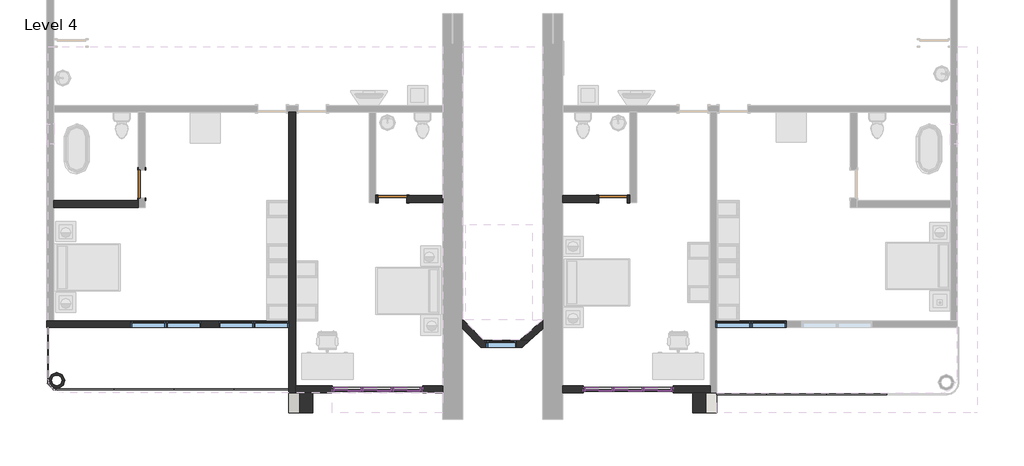
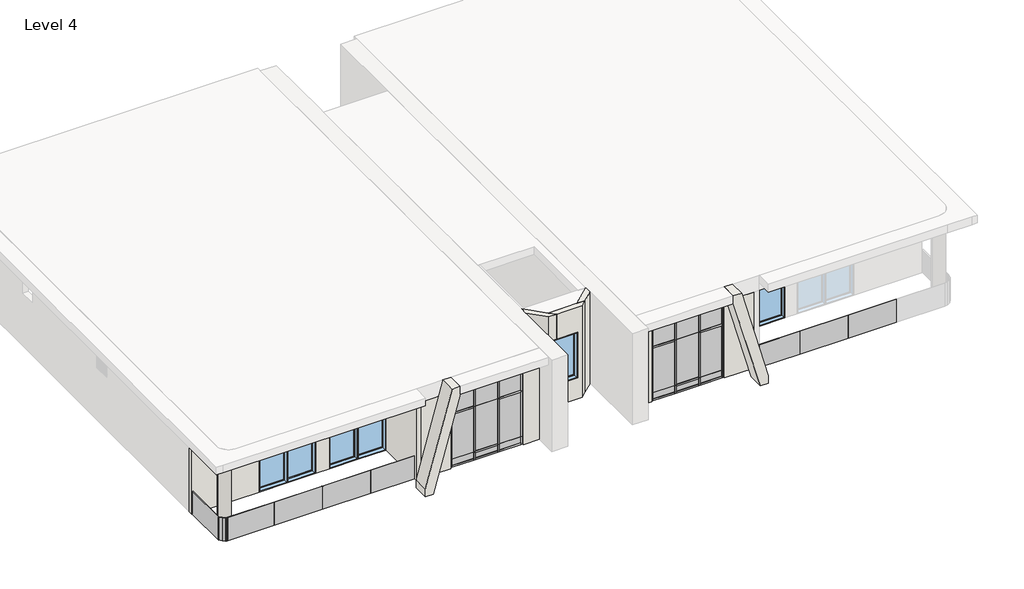
# One storey, part 1 of 3: 42 members, 30 plates, 16 walls, 7 windows, 3 doors.
"""IFC4 building model written with IfcOpenShell, lengths in millimetres."""

from ifc_helpers import new_model, si_unit, point, frame, frame_2d, origin, place, context, project, spatial, polyline, circle_curve, trimmed, segment, composite_curve, outline, extrude, faceted_brep, transform, mapped, element, save
from components import door_2703ae13, door_10fd3a06, member_c17f1be2, member_ad567e07, member_d2e7e466, member_7db1855a, member_75d1e245, member_d60e8053, member_3c3dc66a, member_2fae0574, member_410c6227, member_73c23c35, system_panel_glazed_38d54ecf, system_panel_glazed_fbb6c980, system_panel_glazed_4137532c, system_panel_glazed_6230de04, system_panel_glazed_a79f7f85, system_panel_glazed_9a5ea490, system_panel_glazed_95be5de7, system_panel_glazed_ffe51582, system_panel_glazed_8f95e3f6, system_panel_glazed_836907cd, system_panel_glazed_688a65a2, system_panel_glazed_c1a1c740, system_panel_glazed_22bcd51f, system_panel_glazed_4be86f7f, window_9a779fa2, window_1a213a25

model = new_model("IFC4")

# Units and contexts
model_context = context("Model", 3, world=origin())
ifc_project = project(units=[si_unit("LENGTHUNIT", "METRE", prefix="MILLI")], contexts=[model_context])

# Site, building, storey
site = spatial("IfcSite", under=ifc_project)
building = spatial("IfcBuilding", under=site)
storey = spatial("IfcBuildingStorey", under=building, Name="Level 4", Elevation=10972.8)

# Doors
placement = place(None, origin())
door_shape = door_2703ae13(model_context)
element("IfcDoor", 1, ObjectType="Door-Single-Panel.0001 : 34\" x 80\"", at=placement, inside=storey, context=model_context, shape_type="MappedRepresentation", body=[
    mapped(door_shape, transform((-15765.9987704, -441.9241442, 10972.8), x_axis=(0.0, -1.0, 0.0), y_axis=(1.0, 0.0, 0.0), z_axis=(0.0, 0.0, 1.0))),
])
element("IfcDoor", 2, ObjectType="Door-Single-Panel.0001 : 34\" x 80\"", at=placement, inside=storey, context=model_context, shape_type="MappedRepresentation", body=[
    mapped(door_shape, transform((-8145.9987704, -899.1241442, 10972.8), x_axis=(-1.0, 0.0, 0.0), y_axis=(0.0, -1.0, 0.0), z_axis=(0.0, 0.0, 1.0))),
])
door_2_shape = door_10fd3a06(model_context)
element("IfcDoor", 3, ObjectType="Door-Single-Panel.0001 : 34\" x 80\"", at=placement, inside=storey, context=model_context, shape_type="MappedRepresentation", body=[
    mapped(door_2_shape, transform((-1440.3987704, -899.1241442, 10972.8), x_axis=(1.0, 0.0, 0.0), y_axis=(0.0, 1.0, 0.0), z_axis=(0.0, 0.0, 1.0))),
])

# Members
member_shape = member_c17f1be2(model_context)
element("IfcMember", 4, ObjectType="Rectangular Mullion : 2.5\" x 5\" rectangular", at=placement, inside=storey, context=model_context, shape_type="MappedRepresentation", body=[
    mapped(member_shape, transform((-9911.2987704, -6690.3241442, 14020.8), x_axis=(0.0, 0.0, 1.0), y_axis=(0.0, 1.0, 0.0), z_axis=(-1.0, 0.0, 0.0))),
])
element("IfcMember", 5, ObjectType="Rectangular Mullion : 2.5\" x 5\" rectangular", at=placement, inside=storey, context=model_context, shape_type="MappedRepresentation", body=[
    mapped(member_shape, transform((-8114.2487704, -6690.3241442, 14020.8), x_axis=(0.0, 0.0, 1.0), y_axis=(0.0, 1.0, 0.0), z_axis=(-1.0, 0.0, 0.0))),
])
element("IfcMember", 6, ObjectType="Rectangular Mullion : 2.5\" x 5\" rectangular", at=placement, inside=storey, context=model_context, shape_type="MappedRepresentation", body=[
    mapped(member_shape, transform((-2291.2987704, -6690.3241442, 14020.8), x_axis=(0.0, 0.0, 1.0), y_axis=(0.0, 1.0, 0.0), z_axis=(-1.0, 0.0, 0.0))),
])
element("IfcMember", 7, ObjectType="Rectangular Mullion : 2.5\" x 5\" rectangular", at=placement, inside=storey, context=model_context, shape_type="MappedRepresentation", body=[
    mapped(member_shape, transform((-494.2487704, -6690.3241442, 14020.8), x_axis=(0.0, 0.0, 1.0), y_axis=(0.0, 1.0, 0.0), z_axis=(-1.0, 0.0, 0.0))),
])
element("IfcMember", 8, ObjectType="Rectangular Mullion : 2.5\" x 5\" rectangular", at=placement, inside=storey, context=model_context, shape_type="MappedRepresentation", body=[
    mapped(member_shape, transform((-7295.0987704, -6690.3241442, 10972.8), x_axis=(0.0, 0.0, -1.0), y_axis=(0.0, 1.0, 0.0), z_axis=(1.0, 0.0, 0.0))),
])
element("IfcMember", 9, ObjectType="Rectangular Mullion : 2.5\" x 5\" rectangular", at=placement, inside=storey, context=model_context, shape_type="MappedRepresentation", body=[
    mapped(member_shape, transform((-9092.1487704, -6690.3241442, 10972.8), x_axis=(0.0, 0.0, -1.0), y_axis=(0.0, 1.0, 0.0), z_axis=(1.0, 0.0, 0.0))),
])
element("IfcMember", 10, ObjectType="Rectangular Mullion : 2.5\" x 5\" rectangular", at=placement, inside=storey, context=model_context, shape_type="MappedRepresentation", body=[
    mapped(member_shape, transform((324.9012296, -6690.3241442, 10972.8), x_axis=(0.0, 0.0, -1.0), y_axis=(0.0, 1.0, 0.0), z_axis=(1.0, 0.0, 0.0))),
])
element("IfcMember", 11, ObjectType="Rectangular Mullion : 2.5\" x 5\" rectangular", at=placement, inside=storey, context=model_context, shape_type="MappedRepresentation", body=[
    mapped(member_shape, transform((-1472.1487704, -6690.3241442, 10972.8), x_axis=(0.0, 0.0, -1.0), y_axis=(0.0, 1.0, 0.0), z_axis=(1.0, 0.0, 0.0))),
])
member_2_shape = member_ad567e07(model_context)
element("IfcMember", 12, ObjectType="Rectangular Mullion : 2.5\" x 5\" rectangular", at=placement, inside=storey, context=model_context, shape_type="MappedRepresentation", body=[
    mapped(member_2_shape, transform((-8114.2487704, -6690.3241442, 13106.4), x_axis=(0.0, 0.0, 1.0), y_axis=(0.0, 1.0, 0.0), z_axis=(-1.0, 0.0, 0.0))),
])
element("IfcMember", 13, ObjectType="Rectangular Mullion : 2.5\" x 5\" rectangular", at=placement, inside=storey, context=model_context, shape_type="MappedRepresentation", body=[
    mapped(member_2_shape, transform((-9911.2987704, -6690.3241442, 13106.4), x_axis=(0.0, 0.0, 1.0), y_axis=(0.0, 1.0, 0.0), z_axis=(-1.0, 0.0, 0.0))),
])
element("IfcMember", 14, ObjectType="Rectangular Mullion : 2.5\" x 5\" rectangular", at=placement, inside=storey, context=model_context, shape_type="MappedRepresentation", body=[
    mapped(member_2_shape, transform((-494.2487704, -6690.3241442, 13106.4), x_axis=(0.0, 0.0, 1.0), y_axis=(0.0, 1.0, 0.0), z_axis=(-1.0, 0.0, 0.0))),
])
element("IfcMember", 15, ObjectType="Rectangular Mullion : 2.5\" x 5\" rectangular", at=placement, inside=storey, context=model_context, shape_type="MappedRepresentation", body=[
    mapped(member_2_shape, transform((-2291.2987704, -6690.3241442, 13106.4), x_axis=(0.0, 0.0, 1.0), y_axis=(0.0, 1.0, 0.0), z_axis=(-1.0, 0.0, 0.0))),
])
member_3_shape = member_d2e7e466(model_context)
element("IfcMember", 16, ObjectType="Rectangular Mullion : 2.5\" x 5\" rectangular", at=placement, inside=storey, context=model_context, shape_type="MappedRepresentation", body=[
    mapped(member_3_shape, transform((-8177.7487704, -6690.3241442, 10972.8), x_axis=(0.0, 0.0, -1.0), y_axis=(0.0, 1.0, 0.0), z_axis=(1.0, 0.0, 0.0))),
])
element("IfcMember", 17, ObjectType="Rectangular Mullion : 2.5\" x 5\" rectangular", at=placement, inside=storey, context=model_context, shape_type="MappedRepresentation", body=[
    mapped(member_3_shape, transform((-557.7487704, -6690.3241442, 10972.8), x_axis=(0.0, 0.0, -1.0), y_axis=(0.0, 1.0, 0.0), z_axis=(1.0, 0.0, 0.0))),
])
member_4_shape = member_7db1855a(model_context)
element("IfcMember", 18, ObjectType="Rectangular Mullion : 2.5\" x 5\" rectangular", at=placement, inside=storey, context=model_context, shape_type="MappedRepresentation", body=[
    mapped(member_4_shape, transform((-9028.6487704, -6690.3241442, 11277.6), x_axis=(0.0, 0.0, 1.0), y_axis=(0.0, 1.0, 0.0), z_axis=(-1.0, 0.0, 0.0))),
])
element("IfcMember", 19, ObjectType="Rectangular Mullion : 2.5\" x 5\" rectangular", at=placement, inside=storey, context=model_context, shape_type="MappedRepresentation", body=[
    mapped(member_4_shape, transform((-1408.6487704, -6690.3241442, 11277.6), x_axis=(0.0, 0.0, 1.0), y_axis=(0.0, 1.0, 0.0), z_axis=(-1.0, 0.0, 0.0))),
])
element("IfcMember", 20, ObjectType="Rectangular Mullion : 2.5\" x 5\" rectangular", at=placement, inside=storey, context=model_context, shape_type="MappedRepresentation", body=[
    mapped(member_3_shape, transform((-9028.6487704, -6690.3241442, 14020.8), x_axis=(0.0, 0.0, 1.0), y_axis=(0.0, 1.0, 0.0), z_axis=(-1.0, 0.0, 0.0))),
])
element("IfcMember", 21, ObjectType="Rectangular Mullion : 2.5\" x 5\" rectangular", at=placement, inside=storey, context=model_context, shape_type="MappedRepresentation", body=[
    mapped(member_3_shape, transform((-1408.6487704, -6690.3241442, 14020.8), x_axis=(0.0, 0.0, 1.0), y_axis=(0.0, 1.0, 0.0), z_axis=(-1.0, 0.0, 0.0))),
])
member_5_shape = member_75d1e245(model_context)
element("IfcMember", 22, ObjectType="Rectangular Mullion : 2.5\" x 5\" rectangular", at=placement, inside=storey, context=model_context, shape_type="MappedRepresentation", body=[
    mapped(member_5_shape, transform((-8145.9987704, -6690.3241442, 10972.8), x_axis=(-1.0, 0.0, 0.0), y_axis=(0.0, 1.0, 0.0), z_axis=(0.0, 0.0, -1.0))),
])
element("IfcMember", 23, ObjectType="Rectangular Mullion : 2.5\" x 5\" rectangular", at=placement, inside=storey, context=model_context, shape_type="MappedRepresentation", body=[
    mapped(member_5_shape, transform((-9060.3987704, -6690.3241442, 10972.8), x_axis=(-1.0, 0.0, 0.0), y_axis=(0.0, 1.0, 0.0), z_axis=(0.0, 0.0, -1.0))),
])
element("IfcMember", 24, ObjectType="Rectangular Mullion : 2.5\" x 5\" rectangular", at=placement, inside=storey, context=model_context, shape_type="MappedRepresentation", body=[
    mapped(member_5_shape, transform((-525.9987704, -6690.3241442, 10972.8), x_axis=(-1.0, 0.0, 0.0), y_axis=(0.0, 1.0, 0.0), z_axis=(0.0, 0.0, -1.0))),
])
element("IfcMember", 25, ObjectType="Rectangular Mullion : 2.5\" x 5\" rectangular", at=placement, inside=storey, context=model_context, shape_type="MappedRepresentation", body=[
    mapped(member_5_shape, transform((-1440.3987704, -6690.3241442, 10972.8), x_axis=(-1.0, 0.0, 0.0), y_axis=(0.0, 1.0, 0.0), z_axis=(0.0, 0.0, -1.0))),
])
member_6_shape = member_d60e8053(model_context)
element("IfcMember", 26, ObjectType="Rectangular Mullion : 2.5\" x 5\" rectangular", at=placement, inside=storey, context=model_context, shape_type="MappedRepresentation", body=[
    mapped(member_6_shape, transform((-8145.9987704, -6690.3241442, 11277.6), x_axis=(-1.0, 0.0, 0.0), y_axis=(0.0, 1.0, 0.0), z_axis=(0.0, 0.0, -1.0))),
])
element("IfcMember", 27, ObjectType="Rectangular Mullion : 2.5\" x 5\" rectangular", at=placement, inside=storey, context=model_context, shape_type="MappedRepresentation", body=[
    mapped(member_6_shape, transform((-9060.3987704, -6690.3241442, 11277.6), x_axis=(-1.0, 0.0, 0.0), y_axis=(0.0, 1.0, 0.0), z_axis=(0.0, 0.0, -1.0))),
])
element("IfcMember", 28, ObjectType="Rectangular Mullion : 2.5\" x 5\" rectangular", at=placement, inside=storey, context=model_context, shape_type="MappedRepresentation", body=[
    mapped(member_6_shape, transform((-525.9987704, -6690.3241442, 11277.6), x_axis=(-1.0, 0.0, 0.0), y_axis=(0.0, 1.0, 0.0), z_axis=(0.0, 0.0, -1.0))),
])
element("IfcMember", 29, ObjectType="Rectangular Mullion : 2.5\" x 5\" rectangular", at=placement, inside=storey, context=model_context, shape_type="MappedRepresentation", body=[
    mapped(member_6_shape, transform((-1440.3987704, -6690.3241442, 11277.6), x_axis=(-1.0, 0.0, 0.0), y_axis=(0.0, 1.0, 0.0), z_axis=(0.0, 0.0, -1.0))),
])
member_7_shape = member_3c3dc66a(model_context)
element("IfcMember", 30, ObjectType="Rectangular Mullion : 2.5\" x 5\" rectangular", at=placement, inside=storey, context=model_context, shape_type="MappedRepresentation", body=[
    mapped(member_7_shape, transform((-9974.7987704, -6690.3241442, 10972.8), x_axis=(-1.0, 0.0, 0.0), y_axis=(0.0, 1.0, 0.0), z_axis=(0.0, 0.0, -1.0))),
])
element("IfcMember", 31, ObjectType="Rectangular Mullion : 2.5\" x 5\" rectangular", at=placement, inside=storey, context=model_context, shape_type="MappedRepresentation", body=[
    mapped(member_7_shape, transform((-2354.7987704, -6690.3241442, 10972.8), x_axis=(-1.0, 0.0, 0.0), y_axis=(0.0, 1.0, 0.0), z_axis=(0.0, 0.0, -1.0))),
])
member_8_shape = member_2fae0574(model_context)
element("IfcMember", 32, ObjectType="Rectangular Mullion : 2.5\" x 5\" rectangular", at=placement, inside=storey, context=model_context, shape_type="MappedRepresentation", body=[
    mapped(member_8_shape, transform((-9974.7987704, -6690.3241442, 11277.6), x_axis=(-1.0, 0.0, 0.0), y_axis=(0.0, 1.0, 0.0), z_axis=(0.0, 0.0, -1.0))),
])
element("IfcMember", 33, ObjectType="Rectangular Mullion : 2.5\" x 5\" rectangular", at=placement, inside=storey, context=model_context, shape_type="MappedRepresentation", body=[
    mapped(member_8_shape, transform((-2354.7987704, -6690.3241442, 11277.6), x_axis=(-1.0, 0.0, 0.0), y_axis=(0.0, 1.0, 0.0), z_axis=(0.0, 0.0, -1.0))),
])
element("IfcMember", 34, ObjectType="Rectangular Mullion : 2.5\" x 5\" rectangular", at=placement, inside=storey, context=model_context, shape_type="MappedRepresentation", body=[
    mapped(member_8_shape, transform((-7231.5987704, -6690.3241442, 13106.4), x_axis=(1.0, 0.0, 0.0), y_axis=(0.0, 1.0, 0.0), z_axis=(0.0, 0.0, 1.0))),
])
element("IfcMember", 35, ObjectType="Rectangular Mullion : 2.5\" x 5\" rectangular", at=placement, inside=storey, context=model_context, shape_type="MappedRepresentation", body=[
    mapped(member_8_shape, transform((388.4012296, -6690.3241442, 13106.4), x_axis=(1.0, 0.0, 0.0), y_axis=(0.0, 1.0, 0.0), z_axis=(0.0, 0.0, 1.0))),
])
element("IfcMember", 36, ObjectType="Rectangular Mullion : 2.5\" x 5\" rectangular", at=placement, inside=storey, context=model_context, shape_type="MappedRepresentation", body=[
    mapped(member_7_shape, transform((-7231.5987704, -6690.3241442, 11277.6), x_axis=(1.0, 0.0, 0.0), y_axis=(0.0, 1.0, 0.0), z_axis=(0.0, 0.0, 1.0))),
])
element("IfcMember", 37, ObjectType="Rectangular Mullion : 2.5\" x 5\" rectangular", at=placement, inside=storey, context=model_context, shape_type="MappedRepresentation", body=[
    mapped(member_7_shape, transform((388.4012296, -6690.3241442, 11277.6), x_axis=(1.0, 0.0, 0.0), y_axis=(0.0, 1.0, 0.0), z_axis=(0.0, 0.0, 1.0))),
])
member_9_shape = member_410c6227(model_context)
element("IfcMember", 38, ObjectType="Rectangular Mullion : 2.5\" x 5\" rectangular", at=placement, inside=storey, context=model_context, shape_type="MappedRepresentation", body=[
    mapped(member_9_shape, transform((-8145.9987704, -6690.3241442, 13106.4), x_axis=(-1.0, 0.0, 0.0), y_axis=(0.0, 1.0, 0.0), z_axis=(0.0, 0.0, -1.0))),
])
element("IfcMember", 39, ObjectType="Rectangular Mullion : 2.5\" x 5\" rectangular", at=placement, inside=storey, context=model_context, shape_type="MappedRepresentation", body=[
    mapped(member_9_shape, transform((-9060.3987704, -6690.3241442, 13106.4), x_axis=(-1.0, 0.0, 0.0), y_axis=(0.0, 1.0, 0.0), z_axis=(0.0, 0.0, -1.0))),
])
element("IfcMember", 40, ObjectType="Rectangular Mullion : 2.5\" x 5\" rectangular", at=placement, inside=storey, context=model_context, shape_type="MappedRepresentation", body=[
    mapped(member_9_shape, transform((-525.9987704, -6690.3241442, 13106.4), x_axis=(-1.0, 0.0, 0.0), y_axis=(0.0, 1.0, 0.0), z_axis=(0.0, 0.0, -1.0))),
])
element("IfcMember", 41, ObjectType="Rectangular Mullion : 2.5\" x 5\" rectangular", at=placement, inside=storey, context=model_context, shape_type="MappedRepresentation", body=[
    mapped(member_9_shape, transform((-1440.3987704, -6690.3241442, 13106.4), x_axis=(-1.0, 0.0, 0.0), y_axis=(0.0, 1.0, 0.0), z_axis=(0.0, 0.0, -1.0))),
])
member_10_shape = member_73c23c35(model_context)
element("IfcMember", 42, ObjectType="Rectangular Mullion : 2.5\" x 5\" rectangular", at=placement, inside=storey, context=model_context, shape_type="MappedRepresentation", body=[
    mapped(member_10_shape, transform((-7231.5987704, -6690.3241442, 14020.8), x_axis=(1.0, 0.0, 0.0), y_axis=(0.0, 1.0, 0.0), z_axis=(0.0, 0.0, 1.0))),
])
element("IfcMember", 43, ObjectType="Rectangular Mullion : 2.5\" x 5\" rectangular", at=placement, inside=storey, context=model_context, shape_type="MappedRepresentation", body=[
    mapped(member_10_shape, transform((388.4012296, -6690.3241442, 14020.8), x_axis=(1.0, 0.0, 0.0), y_axis=(0.0, 1.0, 0.0), z_axis=(0.0, 0.0, 1.0))),
])
element("IfcMember", 44, ObjectType="Rectangular Mullion : 2.5\" x 5\" rectangular", at=placement, inside=storey, context=model_context, shape_type="MappedRepresentation", body=[
    mapped(member_10_shape, transform((-9974.7987704, -6690.3241442, 13106.4), x_axis=(-1.0, 0.0, 0.0), y_axis=(0.0, 1.0, 0.0), z_axis=(0.0, 0.0, -1.0))),
])
element("IfcMember", 45, ObjectType="Rectangular Mullion : 2.5\" x 5\" rectangular", at=placement, inside=storey, context=model_context, shape_type="MappedRepresentation", body=[
    mapped(member_10_shape, transform((-2354.7987704, -6690.3241442, 13106.4), x_axis=(-1.0, 0.0, 0.0), y_axis=(0.0, 1.0, 0.0), z_axis=(0.0, 0.0, -1.0))),
])

# Plates
system_panel_glazed_shape = system_panel_glazed_38d54ecf(model_context)
element("IfcPlate", 46, ObjectType="System Panel : Glazed", at=placement, inside=storey, context=model_context, shape_type="MappedRepresentation", body=[
    mapped(system_panel_glazed_shape, transform((-8603.1987704, -6690.3241442, 11309.35), x_axis=(-1.0, 0.0, 0.0), y_axis=(0.0, -1.0, 0.0), z_axis=(0.0, 0.0, 1.0))),
])
element("IfcPlate", 47, ObjectType="System Panel : Glazed", at=placement, inside=storey, context=model_context, shape_type="MappedRepresentation", body=[
    mapped(system_panel_glazed_shape, transform((-983.1987704, -6690.3241442, 11309.35), x_axis=(-1.0, 0.0, 0.0), y_axis=(0.0, -1.0, 0.0), z_axis=(0.0, 0.0, 1.0))),
])
system_panel_glazed_2_shape = system_panel_glazed_fbb6c980(model_context)
element("IfcPlate", 48, ObjectType="System Panel : Glazed", at=placement, inside=storey, context=model_context, shape_type="MappedRepresentation", body=[
    mapped(system_panel_glazed_2_shape, transform((-8603.1987704, -6690.3241442, 11036.3), x_axis=(-1.0, 0.0, 0.0), y_axis=(0.0, -1.0, 0.0), z_axis=(0.0, 0.0, 1.0))),
])
element("IfcPlate", 49, ObjectType="System Panel : Glazed", at=placement, inside=storey, context=model_context, shape_type="MappedRepresentation", body=[
    mapped(system_panel_glazed_2_shape, transform((-983.1987704, -6690.3241442, 11036.3), x_axis=(-1.0, 0.0, 0.0), y_axis=(0.0, -1.0, 0.0), z_axis=(0.0, 0.0, 1.0))),
])
system_panel_glazed_3_shape = system_panel_glazed_4137532c(model_context)
element("IfcPlate", 50, ObjectType="System Panel : Glazed", at=placement, inside=storey, context=model_context, shape_type="MappedRepresentation", body=[
    mapped(system_panel_glazed_3_shape, transform((-7704.6737704, -6690.3241442, 11036.3), x_axis=(-1.0, 0.0, 0.0), y_axis=(0.0, -1.0, 0.0), z_axis=(0.0, 0.0, 1.0))),
])
element("IfcPlate", 51, ObjectType="System Panel : Glazed", at=placement, inside=storey, context=model_context, shape_type="MappedRepresentation", body=[
    mapped(system_panel_glazed_3_shape, transform((-9501.7237704, -6690.3241442, 11036.3), x_axis=(-1.0, 0.0, 0.0), y_axis=(0.0, -1.0, 0.0), z_axis=(0.0, 0.0, 1.0))),
])
element("IfcPlate", 52, ObjectType="System Panel : Glazed", at=placement, inside=storey, context=model_context, shape_type="MappedRepresentation", body=[
    mapped(system_panel_glazed_3_shape, transform((-84.6737704, -6690.3241442, 11036.3), x_axis=(-1.0, 0.0, 0.0), y_axis=(0.0, -1.0, 0.0), z_axis=(0.0, 0.0, 1.0))),
])
element("IfcPlate", 53, ObjectType="System Panel : Glazed", at=placement, inside=storey, context=model_context, shape_type="MappedRepresentation", body=[
    mapped(system_panel_glazed_3_shape, transform((-1881.7237704, -6690.3241442, 11036.3), x_axis=(-1.0, 0.0, 0.0), y_axis=(0.0, -1.0, 0.0), z_axis=(0.0, 0.0, 1.0))),
])
system_panel_glazed_4_shape = system_panel_glazed_6230de04(model_context)
element("IfcPlate", 54, ObjectType="System Panel : Glazed", at=placement, inside=storey, context=model_context, shape_type="MappedRepresentation", body=[
    mapped(system_panel_glazed_4_shape, transform((-7704.6737704, -6690.3241442, 11277.6), x_axis=(-1.0, 0.0, 0.0), y_axis=(0.0, -1.0, 0.0), z_axis=(0.0, 0.0, 1.0))),
])
element("IfcPlate", 55, ObjectType="System Panel : Glazed", at=placement, inside=storey, context=model_context, shape_type="MappedRepresentation", body=[
    mapped(system_panel_glazed_4_shape, transform((-9501.7237704, -6690.3241442, 11277.6), x_axis=(-1.0, 0.0, 0.0), y_axis=(0.0, -1.0, 0.0), z_axis=(0.0, 0.0, 1.0))),
])
element("IfcPlate", 56, ObjectType="System Panel : Glazed", at=placement, inside=storey, context=model_context, shape_type="MappedRepresentation", body=[
    mapped(system_panel_glazed_4_shape, transform((-84.6737704, -6690.3241442, 11277.6), x_axis=(-1.0, 0.0, 0.0), y_axis=(0.0, -1.0, 0.0), z_axis=(0.0, 0.0, 1.0))),
])
element("IfcPlate", 57, ObjectType="System Panel : Glazed", at=placement, inside=storey, context=model_context, shape_type="MappedRepresentation", body=[
    mapped(system_panel_glazed_4_shape, transform((-1881.7237704, -6690.3241442, 11277.6), x_axis=(-1.0, 0.0, 0.0), y_axis=(0.0, -1.0, 0.0), z_axis=(0.0, 0.0, 1.0))),
])
system_panel_glazed_5_shape = system_panel_glazed_a79f7f85(model_context)
element("IfcPlate", 58, ObjectType="System Panel : Glazed", at=placement, inside=storey, context=model_context, shape_type="MappedRepresentation", body=[
    mapped(system_panel_glazed_5_shape, transform((-7704.6737704, -6690.3241442, 13138.15), x_axis=(-1.0, 0.0, 0.0), y_axis=(0.0, -1.0, 0.0), z_axis=(0.0, 0.0, 1.0))),
])
element("IfcPlate", 59, ObjectType="System Panel : Glazed", at=placement, inside=storey, context=model_context, shape_type="MappedRepresentation", body=[
    mapped(system_panel_glazed_5_shape, transform((-9501.7237704, -6690.3241442, 13138.15), x_axis=(-1.0, 0.0, 0.0), y_axis=(0.0, -1.0, 0.0), z_axis=(0.0, 0.0, 1.0))),
])
element("IfcPlate", 60, ObjectType="System Panel : Glazed", at=placement, inside=storey, context=model_context, shape_type="MappedRepresentation", body=[
    mapped(system_panel_glazed_5_shape, transform((-84.6737704, -6690.3241442, 13138.15), x_axis=(-1.0, 0.0, 0.0), y_axis=(0.0, -1.0, 0.0), z_axis=(0.0, 0.0, 1.0))),
])
element("IfcPlate", 61, ObjectType="System Panel : Glazed", at=placement, inside=storey, context=model_context, shape_type="MappedRepresentation", body=[
    mapped(system_panel_glazed_5_shape, transform((-1881.7237704, -6690.3241442, 13138.15), x_axis=(-1.0, 0.0, 0.0), y_axis=(0.0, -1.0, 0.0), z_axis=(0.0, 0.0, 1.0))),
])
system_panel_glazed_6_shape = system_panel_glazed_9a5ea490(model_context)
element("IfcPlate", 62, ObjectType="System Panel : Glazed", at=placement, inside=storey, context=model_context, shape_type="MappedRepresentation", body=[
    mapped(system_panel_glazed_6_shape, transform((-8603.1987704, -6690.3241442, 13106.4), x_axis=(-1.0, 0.0, 0.0), y_axis=(0.0, -1.0, 0.0), z_axis=(0.0, 0.0, 1.0))),
])
element("IfcPlate", 63, ObjectType="System Panel : Glazed", at=placement, inside=storey, context=model_context, shape_type="MappedRepresentation", body=[
    mapped(system_panel_glazed_6_shape, transform((-983.1987704, -6690.3241442, 13106.4), x_axis=(-1.0, 0.0, 0.0), y_axis=(0.0, -1.0, 0.0), z_axis=(0.0, 0.0, 1.0))),
])
system_panel_glazed_7_shape = system_panel_glazed_95be5de7(model_context)
element("IfcPlate", 64, ObjectType="System Panel : Glazed", at=placement, inside=storey, context=model_context, shape_type="MappedRepresentation", body=[
    mapped(system_panel_glazed_7_shape, transform((-15707.2305745, -6723.6923401, 10972.8), x_axis=(1.0, 0.0, 0.0), y_axis=(0.0, 1.0, 0.0), z_axis=(0.0, 0.0, 1.0))),
])
element("IfcPlate", 65, ObjectType="System Panel : Glazed", at=placement, inside=storey, context=model_context, shape_type="MappedRepresentation", body=[
    mapped(system_panel_glazed_7_shape, transform((-13878.4305745, -6723.6923401, 10972.8), x_axis=(1.0, 0.0, 0.0), y_axis=(0.0, 1.0, 0.0), z_axis=(0.0, 0.0, 1.0))),
])
element("IfcPlate", 66, ObjectType="System Panel : Glazed", at=placement, inside=storey, context=model_context, shape_type="MappedRepresentation", body=[
    mapped(system_panel_glazed_7_shape, transform((5957.9120092, -6810.4133646, 10972.8), x_axis=(-1.0, 0.0, 0.0), y_axis=(0.0, -1.0, 0.0), z_axis=(0.0, 0.0, 1.0))),
])
element("IfcPlate", 67, ObjectType="System Panel : Glazed", at=placement, inside=storey, context=model_context, shape_type="MappedRepresentation", body=[
    mapped(system_panel_glazed_7_shape, transform((4129.1120092, -6810.4133646, 10972.8), x_axis=(-1.0, 0.0, 0.0), y_axis=(0.0, -1.0, 0.0), z_axis=(0.0, 0.0, 1.0))),
])
system_panel_glazed_8_shape = system_panel_glazed_ffe51582(model_context)
element("IfcPlate", 68, ObjectType="System Panel : Glazed", at=placement, inside=storey, context=model_context, shape_type="MappedRepresentation", body=[
    mapped(system_panel_glazed_8_shape, transform((-18451.9713429, -6722.1515718, 10972.8), x_axis=(0.7071067811865462, -0.7071067811865488, 0.0), y_axis=(0.7071067811865488, 0.7071067811865462, 0.0), z_axis=(0.0, 0.0, 1.0))),
])
system_panel_glazed_9_shape = system_panel_glazed_8f95e3f6(model_context)
element("IfcPlate", 69, ObjectType="System Panel : Glazed", at=placement, inside=storey, context=model_context, shape_type="MappedRepresentation", body=[
    mapped(system_panel_glazed_9_shape, transform((-18648.8987704, -5667.9741442, 10972.8), x_axis=(0.0, -1.0, 0.0), y_axis=(1.0, 0.0, 0.0), z_axis=(0.0, 0.0, 1.0))),
])
system_panel_glazed_10_shape = system_panel_glazed_836907cd(model_context)
element("IfcPlate", 70, ObjectType="System Panel : Glazed", at=placement, inside=storey, context=model_context, shape_type="MappedRepresentation", body=[
    mapped(system_panel_glazed_10_shape, transform((-18418.6805745, -6723.6923401, 10972.8), x_axis=(1.0, 0.0, 0.0), y_axis=(0.0, 1.0, 0.0), z_axis=(0.0, 0.0, 1.0))),
])
system_panel_glazed_11_shape = system_panel_glazed_688a65a2(model_context)
element("IfcPlate", 71, ObjectType="System Panel : Glazed", at=placement, inside=storey, context=model_context, shape_type="MappedRepresentation", body=[
    mapped(system_panel_glazed_11_shape, transform((-12129.8146725, -6723.6923401, 10972.8), x_axis=(1.0, 0.0, 0.0), y_axis=(0.0, 1.0, 0.0), z_axis=(0.0, 0.0, 1.0))),
])
system_panel_glazed_12_shape = system_panel_glazed_c1a1c740(model_context)
element("IfcPlate", 72, ObjectType="System Panel : Glazed", at=placement, inside=storey, context=model_context, shape_type="MappedRepresentation", body=[
    mapped(system_panel_glazed_12_shape, transform((-17504.2805745, -6723.6923401, 10972.8), x_axis=(1.0, 0.0, 0.0), y_axis=(0.0, 1.0, 0.0), z_axis=(0.0, 0.0, 1.0))),
])
system_panel_glazed_13_shape = system_panel_glazed_22bcd51f(model_context)
element("IfcPlate", 73, ObjectType="System Panel : Glazed", at=placement, inside=storey, context=model_context, shape_type="MappedRepresentation", body=[
    mapped(system_panel_glazed_13_shape, transform((-18600.0521056, -6574.070809, 10972.8), x_axis=(0.7071067811865462, -0.7071067811865488, 0.0), y_axis=(0.7071067811865488, 0.7071067811865462, 0.0), z_axis=(0.0, 0.0, 1.0))),
])
element("IfcPlate", 74, ObjectType="System Panel : Glazed", at=placement, inside=storey, context=model_context, shape_type="MappedRepresentation", body=[
    mapped(system_panel_glazed_13_shape, transform((-18502.3587761, -6671.7641386, 10972.8), x_axis=(0.7071067811865462, -0.7071067811865488, 0.0), y_axis=(0.7071067811865488, 0.7071067811865462, 0.0), z_axis=(0.0, 0.0, 1.0))),
])
system_panel_glazed_14_shape = system_panel_glazed_4be86f7f(model_context)
element("IfcPlate", 75, ObjectType="System Panel : Glazed", at=placement, inside=storey, context=model_context, shape_type="MappedRepresentation", body=[
    mapped(system_panel_glazed_14_shape, transform((2460.5794118, -6810.4133646, 10972.8), x_axis=(-1.0, 0.0, 0.0), y_axis=(0.0, -1.0, 0.0), z_axis=(0.0, 0.0, 1.0))),
])

# Walls
element("IfcWall", 76, ObjectType="Generic - 3\" green 2", at=placement, inside=storey, context=model_context, shape_type="SweptSolid", body=[
    extrude(outline(composite_curve([segment(polyline([(-18518.7237704, -6418.8616442), (-18594.9237704, -6418.8616442)]), True, "CONTINUOUS"), segment(trimmed(circle_curve(frame_2d((-18353.6237704, -6418.8616442)), 241.3), [point((-18594.9237704, -6418.8616442))], [point((-18112.3237704, -6418.8616442))], False, "CARTESIAN"), True, "CONTINUOUS"), segment(polyline([(-18112.3237704, -6418.8616442), (-18188.5237704, -6418.8616442)]), True, "CONTINUOUS"), segment(trimmed(circle_curve(frame_2d((-18353.6237704, -6418.8616442)), 165.1), [point((-18188.5237704, -6418.8616442))], [point((-18518.7237704, -6418.8616442))], True, "CARTESIAN"), True, "CONTINUOUS")], self_intersect=False)), frame((0.0, 0.0, 10972.8), z_axis=(0.0, 0.0, 1.0), x_axis=(1.0, 0.0, 0.0)), (0.0, 0.0, 1.0), 3048.0),
])
element("IfcWall", 77, ObjectType="Generic - 3\" green 2", at=placement, inside=storey, context=model_context, shape_type="SweptSolid", body=[
    extrude(outline(composite_curve([segment(polyline([(-18188.5237704, -6418.8616442), (-18112.3237704, -6418.8616442)]), True, "CONTINUOUS"), segment(trimmed(circle_curve(frame_2d((-18353.6237704, -6418.8616442)), 241.3), [point((-18112.3237704, -6418.8616442))], [point((-18594.9237704, -6418.8616442))], False, "CARTESIAN"), True, "CONTINUOUS"), segment(polyline([(-18594.9237704, -6418.8616442), (-18518.7237704, -6418.8616442)]), True, "CONTINUOUS"), segment(trimmed(circle_curve(frame_2d((-18353.6237704, -6418.8616442)), 165.1), [point((-18518.7237704, -6418.8616442))], [point((-18188.5237704, -6418.8616442))], True, "CARTESIAN"), True, "CONTINUOUS")], self_intersect=False)), frame((0.0, 0.0, 10972.8), z_axis=(0.0, 0.0, 1.0), x_axis=(1.0, 0.0, 0.0)), (0.0, 0.0, 1.0), 3048.0),
])
element("IfcWall", 78, ObjectType="Generic - 8\" cream", at=placement, inside=storey, context=model_context, shape_type="Brep", body=[
    faceted_brep([(-11295.5987704, 1742.4758558, 10972.8), (-11295.5987704, -6791.9241442, 10972.8), (-11295.5987704, -6791.9241442, 14020.8), (-11295.5987704, -4810.7241442, 14020.8), (-11295.5987704, -4607.5241442, 14020.8), (-11295.5987704, 1742.4758558, 14020.8), (-11092.3987704, 1742.4758558, 10972.8), (-11092.3987704, 1742.4758558, 14020.8), (-11092.3987704, -6588.7241442, 14020.8), (-11092.3987704, -6791.9241442, 14020.8), (-11092.3987704, -6791.9241442, 10972.8), (-11092.3987704, -6588.7241442, 10972.8)], [[[0, 1, 2, 3, 4, 5]], [[6, 7, 8, 9, 10, 11]], [[1, 0, 6, 11, 10]], [[5, 4, 3, 2, 9, 8, 7]], [[0, 5, 7, 6]], [[2, 1, 10, 9]]]),
])
element("IfcWall", 79, ObjectType="Generic - 8\" cream", at=placement, inside=storey, context=model_context, shape_type="SweptSolid", body=[
    extrude(outline(polyline([(-18445.6987704, -949.9241442), (-15867.5987704, -949.9241442), (-15867.5987704, -1153.1241442), (-18445.6987704, -1153.1241442), (-18445.6987704, -949.9241442)])), frame((0.0, 0.0, 10972.8), z_axis=(0.0, 0.0, 1.0), x_axis=(1.0, 0.0, 0.0)), (0.0, 0.0, 1.0), 3048.0),
])
element("IfcWall", 80, ObjectType="Generic - 8\" cream", at=placement, inside=storey, context=model_context, shape_type="SweptSolid", body=[
    extrude(outline(polyline([(14020.8, -6621.9987704), (14020.8, -8653.9987704), (10972.8, -8653.9987704), (10972.8, -8577.7987704), (13004.8, -8577.7987704), (13004.8, -7714.1987704), (10972.8, -7714.1987704), (10972.8, -6621.9987704), (14020.8, -6621.9987704)])), frame((0.0, -1000.7241442, 0.0), z_axis=(0.0, 1.0, 0.0), x_axis=(0.0, 0.0, 1.0)), (0.0, 0.0, 1.0), 203.2),
])
element("IfcWall", 81, ObjectType="Generic - 8\" cream", at=placement, inside=storey, context=model_context, shape_type="Brep", body=[
    faceted_brep([(-18648.8987704, -4607.5241442, 14020.8), (-18445.6987704, -4607.5241442, 14020.8), (-11295.5987704, -4607.5241442, 14020.8), (-11295.5987704, -4607.5241442, 13716.0), (-13429.1987704, -4607.5241442, 13716.0), (-13429.1987704, -4607.5241442, 10972.8), (-13962.5987704, -4607.5241442, 10972.8), (-13962.5987704, -4607.5241442, 13716.0), (-16096.1987704, -4607.5241442, 13716.0), (-16096.1987704, -4607.5241442, 10972.8), (-18445.6987704, -4607.5241442, 10972.8), (-18648.8987704, -4607.5241442, 10972.8), (-11295.5987704, -4810.7241442, 14020.8), (-18648.8987704, -4810.7241442, 14020.8), (-18648.8987704, -4810.7241442, 10972.8), (-16096.1987704, -4810.7241442, 10972.8), (-16096.1987704, -4810.7241442, 13716.0), (-13962.5987704, -4810.7241442, 13716.0), (-13962.5987704, -4810.7241442, 10972.8), (-13429.1987704, -4810.7241442, 10972.8), (-13429.1987704, -4810.7241442, 13716.0), (-11295.5987704, -4810.7241442, 13716.0)], [[[0, 1, 2, 3, 4, 5, 6, 7, 8, 9, 10, 11]], [[12, 13, 14, 15, 16, 17, 18, 19, 20, 21]], [[14, 11, 10, 9, 15]], [[5, 19, 18, 6]], [[2, 1, 0, 13, 12]], [[2, 12, 21, 3]], [[0, 11, 14, 13]], [[3, 21, 20, 4]], [[4, 20, 19, 5]], [[17, 7, 6, 18]], [[7, 17, 16, 8]], [[8, 16, 15, 9]]]),
])
element("IfcWall", 82, ObjectType="Generic - 8\" cream", at=placement, inside=storey, context=model_context, shape_type="SweptSolid", body=[
    extrude(outline(polyline([(14020.8, -932.3987704), (14020.8, -2964.3987704), (10972.8, -2964.3987704), (10972.8, -1872.1987704), (13004.8, -1872.1987704), (13004.8, -1008.5987704), (10972.8, -1008.5987704), (10972.8, -932.3987704), (14020.8, -932.3987704)])), frame((0.0, -1000.7241442, 0.0), z_axis=(0.0, 1.0, 0.0), x_axis=(0.0, 0.0, 1.0)), (0.0, 0.0, 1.0), 203.2),
])
element("IfcWall", 83, ObjectType="Generic - 8\" cream", at=placement, inside=storey, context=model_context, shape_type="SweptSolid", body=[
    extrude(outline(polyline([(388.4012296, -6588.7241442), (1506.0012296, -6588.7241442), (1506.0012296, -6791.9241442), (388.4012296, -6791.9241442), (388.4012296, -6588.7241442)])), frame((0.0, 0.0, 10972.8), z_axis=(0.0, 0.0, 1.0), x_axis=(1.0, 0.0, 0.0)), (0.0, 0.0, 1.0), 3048.0),
])
element("IfcWall", 84, ObjectType="Generic - 8\" cream", at=placement, inside=storey, context=model_context, shape_type="SweptSolid", body=[
    extrude(outline(polyline([(-2354.7987704, -6791.9241442), (-2964.3987704, -6791.9241442), (-2964.3987704, -6588.7241442), (-2354.7987704, -6588.7241442), (-2354.7987704, -6791.9241442)])), frame((0.0, 0.0, 10972.8), z_axis=(0.0, 0.0, 1.0), x_axis=(1.0, 0.0, 0.0)), (0.0, 0.0, 1.0), 3048.0),
])
element("IfcWall", 85, ObjectType="Generic - 8\" cream", at=placement, inside=storey, context=model_context, shape_type="SweptSolid", body=[
    extrude(outline(polyline([(-9974.7987704, -6791.9241442), (-11092.3987704, -6791.9241442), (-11092.3987704, -6588.7241442), (-9974.7987704, -6588.7241442), (-9974.7987704, -6791.9241442)])), frame((0.0, 0.0, 10972.8), z_axis=(0.0, 0.0, 1.0), x_axis=(1.0, 0.0, 0.0)), (0.0, 0.0, 1.0), 3048.0),
])
element("IfcWall", 86, ObjectType="Generic - 8\" cream", at=placement, inside=storey, context=model_context, shape_type="SweptSolid", body=[
    extrude(outline(polyline([(-7231.5987704, -6588.7241442), (-6621.9987704, -6588.7241442), (-6621.9987704, -6791.9241442), (-7231.5987704, -6791.9241442), (-7231.5987704, -6588.7241442)])), frame((0.0, 0.0, 10972.8), z_axis=(0.0, 0.0, 1.0), x_axis=(1.0, 0.0, 0.0)), (0.0, 0.0, 1.0), 3048.0),
])
element("IfcWall", 87, ObjectType="Generic - 8\" green", at=placement, inside=storey, context=model_context, shape_type="Brep", body=[
    faceted_brep([(-6012.3987704, -4852.8082422, 10972.8), (-5458.7044276, -5406.502585, 10972.8), (-5458.7044276, -5406.502585, 14630.4), (-6012.3987704, -4852.8082422, 14630.4), (-5171.3362318, -5406.502585, 10972.8), (-5374.5362318, -5203.302585, 10972.8), (-6012.3987704, -4565.4400463, 10972.8), (-6012.3987704, -4565.4400463, 14630.4), (-5374.5362318, -5203.302585, 14630.4), (-5171.3362318, -5406.502585, 14630.4), (-5171.3362318, -5406.502585, 13639.8), (-5289.4901401, -5288.3486766, 13639.8), (-5289.4901401, -5288.3486766, 11811.0), (-5171.3362318, -5406.502585, 11811.0), (-5289.4901401, -5406.502585, 11811.0), (-5289.4901401, -5406.502585, 13639.8)], [[[0, 1, 2, 3]], [[4, 5, 6, 7, 8, 9, 10, 11, 12, 13]], [[1, 0, 6, 5, 4]], [[3, 2, 9, 8, 7]], [[0, 3, 7, 6]], [[2, 1, 4, 13, 14, 15, 10, 9]], [[12, 14, 13]], [[14, 12, 11, 15]], [[15, 11, 10]]]),
])
element("IfcWall", 88, ObjectType="Generic - 8\" green", at=placement, inside=storey, context=model_context, shape_type="Brep", body=[
    faceted_brep([(-5171.3362318, -5406.502585, 10972.8), (-4203.3343712, -5406.502585, 10972.8), (-4203.3343712, -5406.502585, 14630.4), (-5171.3362318, -5406.502585, 14630.4), (-5171.3362318, -5406.502585, 13639.8), (-4375.0901401, -5406.502585, 13639.8), (-4375.0901401, -5406.502585, 11811.0), (-5171.3362318, -5406.502585, 11811.0), (-3975.4820774, -5203.302585, 10972.8), (-4280.7801413, -5203.302585, 10972.8), (-5374.5362318, -5203.302585, 10972.8), (-5374.5362318, -5203.302585, 14630.4), (-4280.7801413, -5203.302585, 14630.4), (-3975.4820774, -5203.302585, 14630.4), (-4375.0901401, -5203.302585, 11811.0), (-4375.0901401, -5203.302585, 13639.8), (-5289.4901401, -5203.302585, 13639.8), (-5289.4901401, -5203.302585, 11811.0), (-5289.4901401, -5288.3486766, 11811.0), (-5289.4901401, -5288.3486766, 13639.8)], [[[0, 1, 2, 3, 4, 5, 6, 7]], [[8, 9, 10, 11, 12, 13], [14, 15, 16, 17]], [[1, 0, 10, 9, 8]], [[3, 2, 13, 12, 11]], [[3, 11, 10, 0, 7, 18, 19, 4]], [[2, 1, 8, 13]], [[5, 15, 14, 6]], [[6, 14, 17, 18, 7]], [[18, 17, 16, 19]], [[15, 5, 4, 19, 16]]]),
])
element("IfcWall", 89, ObjectType="Generic - 8\" green", at=placement, inside=storey, context=model_context, shape_type="SweptSolid", body=[
    extrude(outline(polyline([(-3573.9987704, -4845.2574382), (-3975.4820774, -5203.302585), (-4280.7801413, -5203.302585), (-3573.9987704, -4572.9908503), (-3573.9987704, -4845.2574382)])), frame((0.0, 0.0, 10972.8), z_axis=(0.0, 0.0, 1.0), x_axis=(1.0, 0.0, 0.0)), (0.0, 0.0, 1.0), 3657.6),
])
element("IfcWall", 90, ObjectType="Generic -2' white 2", at=placement, inside=storey, context=model_context, shape_type="SweptSolid", body=[
    extrude(outline(polyline([(14325.6, -9974.7987704), (14630.4, -9974.7987704), (14630.4, -10279.5987704), (10972.8, -11295.5987704), (10668.0, -11295.5987704), (10668.0, -10990.7987704), (14325.6, -9974.7987704)])), frame((0.0, -7401.5241442, 0.0), z_axis=(0.0, 1.0, 0.0), x_axis=(0.0, 0.0, 1.0)), (0.0, 0.0, 1.0), 609.6),
])
element("IfcWall", 91, ObjectType="Generic -2' white 2", at=placement, inside=storey, context=model_context, shape_type="SweptSolid", body=[
    extrude(outline(polyline([(14325.6, 385.6468143), (10668.0, 1401.6468143), (10668.0, 1706.4468143), (10972.8, 1706.4468143), (14630.4, 690.4468143), (14630.4, 385.6468143), (14325.6, 385.6468143)])), frame((0.0, -7401.5241442, 0.0), z_axis=(0.0, 1.0, 0.0), x_axis=(0.0, 0.0, 1.0)), (0.0, 0.0, 1.0), 609.6),
])

# Windows
window_shape = window_9a779fa2(model_context)
element("IfcWindow", 92, ObjectType="Fixed : 36\" x 72\"", at=placement, inside=storey, context=model_context, shape_type="MappedRepresentation", body=[
    mapped(window_shape, transform((-4794.1901401, -5304.902585, 11506.2), x_axis=(1.0, 0.0, 0.0), y_axis=(0.0, 1.0, 0.0), z_axis=(0.0, 0.0, 1.0))),
])
window_2_shape = window_1a213a25(model_context)
element("IfcWindow", 93, ObjectType="Fixed : 36\" x 72\" 2", at=placement, inside=storey, context=model_context, shape_type="MappedRepresentation", body=[
    mapped(window_2_shape, transform((-11790.8987704, -4709.1241442, 10668.0), x_axis=(1.0, 0.0, 0.0), y_axis=(0.0, 1.0, 0.0), z_axis=(0.0, 0.0, 1.0))),
])
element("IfcWindow", 94, ObjectType="Fixed : 36\" x 72\" 2", at=placement, inside=storey, context=model_context, shape_type="MappedRepresentation", body=[
    mapped(window_2_shape, transform((-12857.6987704, -4709.1241442, 10668.0), x_axis=(1.0, 0.0, 0.0), y_axis=(0.0, 1.0, 0.0), z_axis=(0.0, 0.0, 1.0))),
])
element("IfcWindow", 95, ObjectType="Fixed : 36\" x 72\" 2", at=placement, inside=storey, context=model_context, shape_type="MappedRepresentation", body=[
    mapped(window_2_shape, transform((-14457.8987704, -4709.1241442, 10668.0), x_axis=(1.0, 0.0, 0.0), y_axis=(0.0, 1.0, 0.0), z_axis=(0.0, 0.0, 1.0))),
])
element("IfcWindow", 96, ObjectType="Fixed : 36\" x 72\" 2", at=placement, inside=storey, context=model_context, shape_type="MappedRepresentation", body=[
    mapped(window_2_shape, transform((-15524.6987704, -4709.1241442, 10668.0), x_axis=(1.0, 0.0, 0.0), y_axis=(0.0, 1.0, 0.0), z_axis=(0.0, 0.0, 1.0))),
])
element("IfcWindow", 97, ObjectType="Fixed : 36\" x 72\" 2", at=placement, inside=storey, context=model_context, shape_type="MappedRepresentation", body=[
    mapped(window_2_shape, transform((2255.3012296, -4709.1241442, 10668.0), x_axis=(1.0, 0.0, 0.0), y_axis=(0.0, 1.0, 0.0), z_axis=(0.0, 0.0, 1.0))),
])
element("IfcWindow", 98, ObjectType="Fixed : 36\" x 72\" 2", at=placement, inside=storey, context=model_context, shape_type="MappedRepresentation", body=[
    mapped(window_2_shape, transform((3331.6262296, -4709.1241442, 10668.0), x_axis=(1.0, 0.0, 0.0), y_axis=(0.0, 1.0, 0.0), z_axis=(0.0, 0.0, 1.0))),
])

save(model, "model.ifc")

# Revit data of these elements
# Type "Door-Single-Panel.0001 : 34\" x 80\""
#   Type Mark = "9"
#   Construction Type Id = "DOOR"
#   Assembly Code = "C1020300"
#   Analytic Construction = "Wooden"
#   Thickness = 0' - 2"
#   Thermal Resistance (R) = 0.455703 (m²·K)/W
#   Swing Angle [instance default] = 90.00°
#   Heat Transfer Coefficient (U) = 2.19465 W/(m²·K)
#   Height = 6' - 8"
#   Trim Projection Ext = 0' - 1"
#   Trim Projection Int = 0' - 1"
#   Trim Width = 0' - 3"
#   Width = 2' - 10"
#   Panel Material = Wood - Birch - Solid Stained Light Low Gloss
#   Trim Material = Paint - Sienna
#   Visual Light Transmittance = 0
#   Solar Heat Gain Coefficient = 0
#   Function = (empty or 0)
#   Wall Closure = (empty or 0)
# Type "Rectangular Mullion : 2.5\" x 5\" rectangular"
#   built-in parameter 1007304 = 0.416667 (stored number, unit not read)
#   built-in parameter 1007301 = 0.104167 (stored number, unit not read)
#   built-in parameter 1007300 = 0.104167 (stored number, unit not read)
# Type "System Panel : Glazed"
#   Construction Type Id = "GSP4R"
#   Analytic Construction = "1/8 in Pilkington single glazing"
#   Visual Light Transmittance = 0.9
#   Solar Heat Gain Coefficient = 0.86
#   Heat Transfer Coefficient (U) = 6.7069 W/(m²·K)
# Type "Generic - 3\" green 2"
#   Assembly Code = "B2010"
#   Width = 0' - 3"
#   Layers, outside or top first: 0' - 3" "Damp-proofing" (function 1)
# Type "Generic - 8\" cream"
#   Assembly Code = "B2010"
#   Width = 0' - 8"
#   Layers, outside or top first: 0' - 8" "Parking Stripe" (function 1)
# Type "Generic - 8\" green"
#   Assembly Code = "B2010"
#   Width = 0' - 8"
#   Layers, outside or top first: 0' - 8" "Damp-proofing" (function 1)
# Type "Generic -2' white 2"
#   Assembly Code = "B2010"
#   Width = 2' - 0"
#   Layers, outside or top first: 2' - 0" "Door - Frame" (function 1)
# Type "Fixed : 36\" x 72\""
#   Type Mark = "9"
#   Construction Type Id = "GSP4R"
#   Assembly Code = "B2020100"
#   Analytic Construction = "1/8 in Pilkington single glazing"
#   Visual Light Transmittance = 0.9
#   Solar Heat Gain Coefficient = 0.78
#   Heat Transfer Coefficient (U) = 3.6886 W/(m²·K)
#   Height = 6' - 0"
#   Default Sill Height = 1' - 0"
#   Width = 3' - 0"
#   Window Inset = 0' - 0 3/4"
#   Glass Pane Material = Glass
#   Sash Material = Iron, Ductile
#   Wall Closure = (empty or 0)
# Type "Fixed : 36\" x 72\" 2"
#   Type Mark = "29"
#   Construction Type Id = "GSP4R"
#   Assembly Code = "B2020100"
#   Analytic Construction = "1/8 in Pilkington single glazing"
#   Visual Light Transmittance = 0.9
#   Solar Heat Gain Coefficient = 0.78
#   Heat Transfer Coefficient (U) = 3.6886 W/(m²·K)
#   Height = 9' - 0"
#   Default Sill Height = 1' - 0"
#   Width = 3' - 6"
#   Window Inset = 0' - 0 3/4"
#   Glass Pane Material = Glass
#   Sash Material = Iron, Ductile
#   Wall Closure = (empty or 0)
# Elements 1, 2, 3 (IfcDoor, "Door-Single-Panel.0001 : 34\" x 80\"")
#   Swing Angle = 90.00°
#   Phase Created = New Construction
#   Materials on its faces: "Paint - Sienna", "Wood - Birch - Solid Stained Light Low Gloss"
# Elements 4, 5, 6, 7, 8, 9, 10, 11, 12, 13, 14, 15, 16, 17, 18, 19, 20, 21, 22, 23, 24, 25, 26, 27, 28, 29, 30, 31, 32, 33, 34, 35, 36, 37, 38, 39, 40, 41, 42, 43, 44, 45 (IfcMember, "Rectangular Mullion : 2.5\" x 5\" rectangular")
#   Phase Created = New Construction
#   Materials on its faces: "Iron, Ductile"
# Elements 46, 47, 48, 49, 50, 51, 52, 53, 54, 55, 56, 57, 58, 59, 60, 61, 62, 63, 64, 65, 66, 67, 68, 69, 70, 71, 72, 73, 74, 75 (IfcPlate, "System Panel : Glazed")
#   Phase Created = New Construction
#   Materials on its faces: "Glass"
# Elements 76, 77 (IfcWall, "Generic - 3\" green 2")
#   Top Offset = 0' - 0"
#   Base Offset = 0' - 0"
#   Unconnected Height = 10' - 0"
#   wall height = 10' - 0"
#   Phase Created = New Construction
#   Materials on its faces: "Damp-proofing"
# Elements 78, 79, 80, 81, 82, 83, 84, 85, 86 (IfcWall, "Generic - 8\" cream")
#   Top Offset = 0' - 0"
#   Base Offset = 0' - 0"
#   Unconnected Height = 10' - 0"
#   wall height = 10' - 0"
#   Phase Created = New Construction
#   Base Constraint = Level 4
#   Materials on its faces: "Parking Stripe"
# Elements 87, 88, 89 (IfcWall, "Generic - 8\" green")
#   Top Offset = 0' - 0"
#   Base Offset = 0' - 0"
#   Unconnected Height = 12' - 0"
#   wall height = 12' - 0"
#   Phase Created = New Construction
#   Base Constraint = Level 4
#   Materials on its faces: "Damp-proofing"
# Elements 90, 91 (IfcWall, "Generic -2' white 2")
#   built-in parameter 1001111 = -1' - 0"
#   Top Offset = 0' - 0"
#   Base Offset = -1' - 0"
#   Unconnected Height = 13' - 0"
#   wall height = 13' - 0"
#   Phase Created = New Construction
#   Base Constraint = Level 4
#   Materials on its faces: "Door - Frame"
# Element 92 (IfcWindow, "Fixed : 36\" x 72\"")
#   Mark = "112"
#   Phase Created = New Construction
#   Materials on its faces: "Iron, Ductile", "Glass"
# Element 93 (IfcWindow, "Fixed : 36\" x 72\" 2")
#   Mark = "113"
#   Phase Created = New Construction
#   Materials on its faces: "Iron, Ductile", "Glass"
# Element 94 (IfcWindow, "Fixed : 36\" x 72\" 2")
#   Mark = "114"
#   Phase Created = New Construction
#   Materials on its faces: "Iron, Ductile", "Glass"
# Element 95 (IfcWindow, "Fixed : 36\" x 72\" 2")
#   Mark = "115"
#   Phase Created = New Construction
#   Materials on its faces: "Iron, Ductile", "Glass"
# Element 96 (IfcWindow, "Fixed : 36\" x 72\" 2")
#   Mark = "116"
#   Phase Created = New Construction
#   Materials on its faces: "Iron, Ductile", "Glass"
# Element 97 (IfcWindow, "Fixed : 36\" x 72\" 2")
#   Mark = "117"
#   Phase Created = New Construction
#   Materials on its faces: "Iron, Ductile", "Glass"
# Element 98 (IfcWindow, "Fixed : 36\" x 72\" 2")
#   Mark = "118"
#   Phase Created = New Construction
#   Materials on its faces: "Iron, Ductile", "Glass"
# Materials
#   "Wood - Birch - Solid Stained Light Low Gloss": class "Wood", colour RGB 210 159 95, transparency 0, Cost = 0
#   "Paint - Sienna": colour RGB 118 70 51, transparency 0, Cost = 0
#   "Damp-proofing": class "Generic", colour RGB 127 127 127, transparency 0, Description = "Damp-proofing", Cost = 0
#   "Parking Stripe": class "Paint", colour RGB 250 250 91, transparency 0, Cost = 0
#   "Door - Frame": colour RGB 118 70 51, transparency 0, Cost = 0
#   "Glass": class "Glass", colour RGB 0 128 192, transparency 0.75, Description = "Soda Lime Glass", Cost = 0
#   "Iron, Ductile": class "Metal", colour RGB 0 0 0, transparency 0, Description = "Ductile cast iron", Cost = 0
